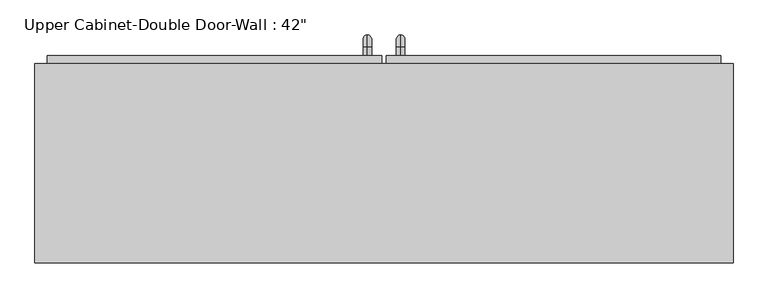
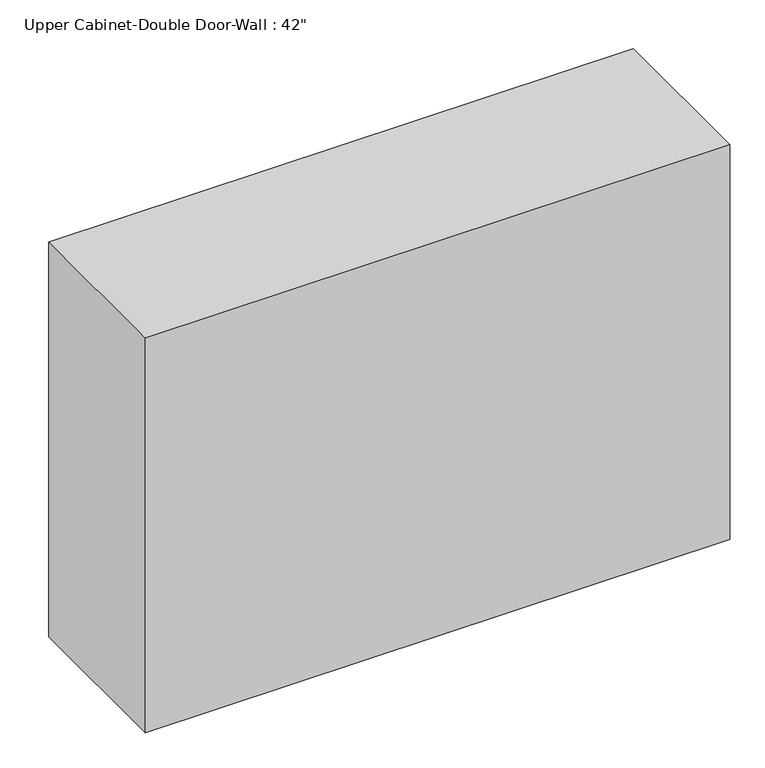
"""IFC4 building model written with IfcOpenShell, lengths in millimetres: furniture geometry."""

from ifc_helpers import new_model, si_unit, point, frame, origin, place, context, project, spatial, polyline, circle_curve, ellipse_curve, trimmed, outline, extrude, faceted_brep, source, transform, mapped, element, save
from ifc_brep_helpers import plane_surface, cylinder_surface, revolved_surface, advanced_brep


def furniture_7e2871f8(model_context):
    return source(origin(), model_context, "Body", "SolidModel", [
        faceted_brep([(-503.6288372, 101.6, 2133.6), (-503.6288372, 101.6, 1371.6), (563.1711628, 101.6, 1371.6), (563.1711628, 101.6, 2133.6), (-503.6288372, 406.4, 2133.6), (563.1711628, 406.4, 2133.6), (563.1711628, 406.4, 1371.6), (-503.6288372, 406.4, 1371.6), (-484.5788372, 406.4, 2114.55), (-484.5788372, 406.4, 1390.65), (544.1211628, 406.4, 1390.65), (544.1211628, 406.4, 2114.55), (544.1211628, 120.65, 2114.55), (-484.5788372, 120.65, 2114.55), (544.1211628, 120.65, 1390.65), (-484.5788372, 120.65, 1390.65)], [[[0, 1, 2, 3]], [[4, 5, 6, 7], [8, 9, 10, 11]], [[1, 0, 4, 7]], [[2, 1, 7, 6]], [[3, 2, 6, 5]], [[0, 3, 5, 4]], [[8, 11, 12, 13]], [[11, 10, 14, 12]], [[10, 9, 15, 14]], [[9, 8, 13, 15]], [[13, 12, 14, 15]]]),
        advanced_brep(
        [(55.1711628, 419.1, 1517.65), (55.1711628, 419.1, 1530.35), (55.1711628, 431.8, 1517.65), (55.1711628, 431.8, 1530.35), (55.1711628, 450.85, 1511.3), (55.1711628, 438.15, 1511.3), (55.1711628, 438.15, 1435.1), (55.1711628, 450.85, 1435.1), (55.1711628, 431.8, 1416.05), (55.1711628, 431.8, 1428.75), (55.1711628, 419.1, 1428.75), (55.1711628, 419.1, 1416.05)],
        [
            (0, 1, circle_curve(frame((55.1711628, 419.1, 1524.0), z_axis=(0.0, -1.0, 0.0), x_axis=(0.0, 0.0, -1.0)), 6.35)),
            (1, 0, circle_curve(frame((55.1711628, 419.1, 1524.0), z_axis=(0.0, -1.0, 0.0), x_axis=(0.0, 0.0, -1.0)), 6.35)),
            (0, 2),
            (2, 3, circle_curve(frame((55.1711628, 431.8, 1524.0), z_axis=(0.0, -1.0, 0.0), x_axis=(0.0, 0.0, -1.0)), 6.35)),
            (3, 1),
            (3, 2, circle_curve(frame((55.1711628, 431.8, 1524.0), z_axis=(0.0, -1.0, 0.0), x_axis=(0.0, 0.0, -1.0)), 6.35)),
            (4, 3, circle_curve(frame((55.1711628, 431.8, 1511.3), z_axis=(1.0, 0.0, 0.0), x_axis=(0.0, 0.0, 1.0)), 19.05)),
            (2, 5, circle_curve(frame((55.1711628, 431.8, 1511.3), z_axis=(-1.0, 0.0, 0.0), x_axis=(0.0, 0.0, 1.0)), 6.35)),
            (5, 4, circle_curve(frame((55.1711628, 444.5, 1511.3), z_axis=(0.0, 0.0, 1.0), x_axis=(0.0, -1.0, 0.0)), 6.35)),
            (4, 5, circle_curve(frame((55.1711628, 444.5, 1511.3), z_axis=(0.0, 0.0, 1.0), x_axis=(0.0, -1.0, 0.0)), 6.35)),
            (5, 6),
            (6, 7, circle_curve(frame((55.1711628, 444.5, 1435.1), z_axis=(0.0, 0.0, 1.0), x_axis=(0.0, -1.0, 0.0)), 6.35)),
            (7, 4),
            (7, 6, circle_curve(frame((55.1711628, 444.5, 1435.1), z_axis=(0.0, 0.0, 1.0), x_axis=(0.0, -1.0, 0.0)), 6.35)),
            (8, 7, circle_curve(frame((55.1711628, 431.8, 1435.1), z_axis=(1.0, 0.0, 0.0), x_axis=(0.0, 1.0, 0.0)), 19.05)),
            (6, 9, circle_curve(frame((55.1711628, 431.8, 1435.1), z_axis=(-1.0, 0.0, 0.0), x_axis=(0.0, 1.0, 0.0)), 6.35)),
            (9, 8, circle_curve(frame((55.1711628, 431.8, 1422.4), z_axis=(0.0, 1.0, 0.0), x_axis=(0.0, 0.0, 1.0)), 6.35)),
            (8, 9, circle_curve(frame((55.1711628, 431.8, 1422.4), z_axis=(0.0, 1.0, 0.0), x_axis=(0.0, 0.0, 1.0)), 6.35)),
            (10, 11, circle_curve(frame((55.1711628, 419.1, 1422.4), z_axis=(0.0, -1.0, 0.0), x_axis=(0.0, 0.0, 1.0)), 6.35)),
            (11, 10, circle_curve(frame((55.1711628, 419.1, 1422.4), z_axis=(0.0, -1.0, 0.0), x_axis=(0.0, 0.0, 1.0)), 6.35)),
            (9, 10),
            (11, 8),
        ],
        [
            plane_surface(frame((48.8211628, 419.1, 1524.0), z_axis=(0.0, -1.0, 0.0), x_axis=(0.0, 0.0, 1.0))),
            cylinder_surface(frame((55.1711628, 419.1, 1524.0), z_axis=(0.0, -1.0, 0.0), x_axis=(0.0, 0.0, -1.0)), 6.35),
            revolved_surface(trimmed(ellipse_curve(frame((55.1711628, 431.8, 1524.0), z_axis=(0.0, -1.0, 0.0), x_axis=(0.0, 0.0, -1.0)), 6.35, 6.35), [point((55.1711628, 431.8, 1517.65))], [point((55.1711628, 431.8, 1530.35))], True, "CARTESIAN"), (55.1711628, 431.8, 1511.3), (-1.0, 0.0, 0.0)),
            revolved_surface(trimmed(ellipse_curve(frame((55.1711628, 431.8, 1524.0), z_axis=(0.0, -1.0, 0.0), x_axis=(0.0, 0.0, -1.0)), 6.35, 6.35), [point((55.1711628, 431.8, 1530.35))], [point((55.1711628, 431.8, 1517.65))], True, "CARTESIAN"), (55.1711628, 431.8, 1511.3), (-1.0, 0.0, 0.0)),
            cylinder_surface(frame((55.1711628, 444.5, 1511.3), z_axis=(0.0, 0.0, 1.0), x_axis=(0.0, -1.0, 0.0)), 6.35),
            revolved_surface(trimmed(ellipse_curve(frame((55.1711628, 444.5, 1435.1), z_axis=(0.0, 0.0, 1.0), x_axis=(0.0, -1.0, 0.0)), 6.35, 6.35), [point((55.1711628, 438.15, 1435.1))], [point((55.1711628, 450.85, 1435.1))], True, "CARTESIAN"), (55.1711628, 431.8, 1435.1), (-1.0, 0.0, 0.0)),
            revolved_surface(trimmed(ellipse_curve(frame((55.1711628, 444.5, 1435.1), z_axis=(0.0, 0.0, 1.0), x_axis=(0.0, -1.0, 0.0)), 6.35, 6.35), [point((55.1711628, 450.85, 1435.1))], [point((55.1711628, 438.15, 1435.1))], True, "CARTESIAN"), (55.1711628, 431.8, 1435.1), (-1.0, 0.0, 0.0)),
            plane_surface(frame((48.8211628, 419.1, 1422.4), z_axis=(0.0, -1.0, 0.0), x_axis=(0.0, 0.0, -1.0))),
            cylinder_surface(frame((55.1711628, 431.8, 1422.4), z_axis=(0.0, 1.0, 0.0), x_axis=(0.0, 0.0, 1.0)), 6.35),
        ],
        [
            (0, [[1, 2]]),
            (1, [[-1, 3, 4, 5]]),
            (1, [[-2, -5, 6, -3]]),
            (2, [[7, -4, 8, 9]]),
            (3, [[-8, -6, -7, 10]]),
            (4, [[-9, 11, 12, 13]]),
            (4, [[-10, -13, 14, -11]]),
            (5, [[15, -12, 16, 17]]),
            (6, [[-16, -14, -15, 18]]),
            (7, [[19, 20]]),
            (8, [[-17, 21, -20, 22]]),
            (8, [[-18, -22, -19, -21]]),
        ],
    ),
        advanced_brep(
        [(4.3711628, 419.1, 1517.65), (4.3711628, 419.1, 1530.35), (4.3711628, 431.8, 1517.65), (4.3711628, 431.8, 1530.35), (4.3711628, 450.85, 1511.3), (4.3711628, 438.15, 1511.3), (4.3711628, 438.15, 1435.1), (4.3711628, 450.85, 1435.1), (4.3711628, 431.8, 1416.05), (4.3711628, 431.8, 1428.75), (4.3711628, 419.1, 1428.75), (4.3711628, 419.1, 1416.05)],
        [
            (0, 1, circle_curve(frame((4.3711628, 419.1, 1524.0), z_axis=(0.0, -1.0, 0.0), x_axis=(0.0, 0.0, 1.0)), 6.35)),
            (1, 0, circle_curve(frame((4.3711628, 419.1, 1524.0), z_axis=(0.0, -1.0, 0.0), x_axis=(0.0, 0.0, 1.0)), 6.35)),
            (0, 2),
            (2, 3, circle_curve(frame((4.3711628, 431.8, 1524.0), z_axis=(0.0, -1.0, 0.0), x_axis=(0.0, 0.0, 1.0)), 6.35)),
            (3, 1),
            (3, 2, circle_curve(frame((4.3711628, 431.8, 1524.0), z_axis=(0.0, -1.0, 0.0), x_axis=(0.0, 0.0, 1.0)), 6.35)),
            (4, 3, circle_curve(frame((4.3711628, 431.8, 1511.3), z_axis=(1.0, 0.0, 0.0), x_axis=(0.0, 0.0, 1.0)), 19.05)),
            (2, 5, circle_curve(frame((4.3711628, 431.8, 1511.3), z_axis=(-1.0, 0.0, 0.0), x_axis=(0.0, 0.0, 1.0)), 6.35)),
            (5, 4, circle_curve(frame((4.3711628, 444.5, 1511.3), z_axis=(0.0, 0.0, 1.0), x_axis=(0.0, 1.0, 0.0)), 6.35)),
            (4, 5, circle_curve(frame((4.3711628, 444.5, 1511.3), z_axis=(0.0, 0.0, 1.0), x_axis=(0.0, 1.0, 0.0)), 6.35)),
            (5, 6),
            (6, 7, circle_curve(frame((4.3711628, 444.5, 1435.1), z_axis=(0.0, 0.0, 1.0), x_axis=(0.0, 1.0, 0.0)), 6.35)),
            (7, 4),
            (7, 6, circle_curve(frame((4.3711628, 444.5, 1435.1), z_axis=(0.0, 0.0, 1.0), x_axis=(0.0, 1.0, 0.0)), 6.35)),
            (8, 7, circle_curve(frame((4.3711628, 431.8, 1435.1), z_axis=(1.0, 0.0, 0.0), x_axis=(0.0, 1.0, 0.0)), 19.05)),
            (6, 9, circle_curve(frame((4.3711628, 431.8, 1435.1), z_axis=(-1.0, 0.0, 0.0), x_axis=(0.0, 1.0, 0.0)), 6.35)),
            (9, 8, circle_curve(frame((4.3711628, 431.8, 1422.4), z_axis=(0.0, 1.0, 0.0), x_axis=(0.0, 0.0, -1.0)), 6.35)),
            (8, 9, circle_curve(frame((4.3711628, 431.8, 1422.4), z_axis=(0.0, 1.0, 0.0), x_axis=(0.0, 0.0, -1.0)), 6.35)),
            (10, 11, circle_curve(frame((4.3711628, 419.1, 1422.4), z_axis=(0.0, -1.0, 0.0), x_axis=(0.0, 0.0, -1.0)), 6.35)),
            (11, 10, circle_curve(frame((4.3711628, 419.1, 1422.4), z_axis=(0.0, -1.0, 0.0), x_axis=(0.0, 0.0, -1.0)), 6.35)),
            (9, 10),
            (11, 8),
        ],
        [
            plane_surface(frame((-1.9788372, 419.1, 1524.0), z_axis=(0.0, -1.0, 0.0), x_axis=(0.0, 0.0, 1.0))),
            cylinder_surface(frame((4.3711628, 419.1, 1524.0), z_axis=(0.0, -1.0, 0.0), x_axis=(0.0, 0.0, 1.0)), 6.35),
            revolved_surface(trimmed(ellipse_curve(frame((4.3711628, 431.8, 1524.0), z_axis=(0.0, -1.0, 0.0), x_axis=(0.0, 0.0, 1.0)), 6.35, 6.35), [point((4.3711628, 431.8, 1517.65))], [point((4.3711628, 431.8, 1530.35))], True, "CARTESIAN"), (4.3711628, 431.8, 1511.3), (-1.0, 0.0, 0.0)),
            revolved_surface(trimmed(ellipse_curve(frame((4.3711628, 431.8, 1524.0), z_axis=(0.0, -1.0, 0.0), x_axis=(0.0, 0.0, 1.0)), 6.35, 6.35), [point((4.3711628, 431.8, 1530.35))], [point((4.3711628, 431.8, 1517.65))], True, "CARTESIAN"), (4.3711628, 431.8, 1511.3), (-1.0, 0.0, 0.0)),
            cylinder_surface(frame((4.3711628, 444.5, 1511.3), z_axis=(0.0, 0.0, 1.0), x_axis=(0.0, 1.0, 0.0)), 6.35),
            revolved_surface(trimmed(ellipse_curve(frame((4.3711628, 444.5, 1435.1), z_axis=(0.0, 0.0, 1.0), x_axis=(0.0, 1.0, 0.0)), 6.35, 6.35), [point((4.3711628, 438.15, 1435.1))], [point((4.3711628, 450.85, 1435.1))], True, "CARTESIAN"), (4.3711628, 431.8, 1435.1), (-1.0, 0.0, 0.0)),
            revolved_surface(trimmed(ellipse_curve(frame((4.3711628, 444.5, 1435.1), z_axis=(0.0, 0.0, 1.0), x_axis=(0.0, 1.0, 0.0)), 6.35, 6.35), [point((4.3711628, 450.85, 1435.1))], [point((4.3711628, 438.15, 1435.1))], True, "CARTESIAN"), (4.3711628, 431.8, 1435.1), (-1.0, 0.0, 0.0)),
            plane_surface(frame((-1.9788372, 419.1, 1422.4), z_axis=(0.0, -1.0, 0.0), x_axis=(0.0, 0.0, -1.0))),
            cylinder_surface(frame((4.3711628, 431.8, 1422.4), z_axis=(0.0, 1.0, 0.0), x_axis=(0.0, 0.0, -1.0)), 6.35),
        ],
        [
            (0, [[1, 2]]),
            (1, [[-1, 3, 4, 5]]),
            (1, [[-2, -5, 6, -3]]),
            (2, [[7, -4, 8, 9]]),
            (3, [[-8, -6, -7, 10]]),
            (4, [[-9, 11, 12, 13]]),
            (4, [[-10, -13, 14, -11]]),
            (5, [[15, -12, 16, 17]]),
            (6, [[-16, -14, -15, 18]]),
            (7, [[19, 20]]),
            (8, [[-17, 21, -20, 22]]),
            (8, [[-18, -22, -19, -21]]),
        ],
    ),
        extrude(outline(polyline([(32.9461628, 419.1), (544.1211628, 419.1), (544.1211628, 387.35), (32.9461628, 387.35), (32.9461628, 419.1)])), frame((0.0, 0.0, 1390.65), z_axis=(0.0, 0.0, 1.0), x_axis=(1.0, 0.0, 0.0)), (0.0, 0.0, 1.0), 723.9),
        extrude(outline(polyline([(-484.5788372, 419.1), (26.5961628, 419.1), (26.5961628, 387.35), (-484.5788372, 387.35), (-484.5788372, 419.1)])), frame((0.0, 0.0, 1390.65), z_axis=(0.0, 0.0, 1.0), x_axis=(1.0, 0.0, 0.0)), (0.0, 0.0, 1.0), 723.9),
    ])


if __name__ == "__main__":
    model = new_model("IFC4")
    model_context = context("Model", 3, world=origin())
    ifc_project = project(units=[si_unit("LENGTHUNIT", "METRE", prefix="MILLI")], contexts=[model_context])
    site = spatial("IfcSite", under=ifc_project)
    building = spatial("IfcBuilding", under=site)
    placement = place(None, origin())
    furniture_shape = furniture_7e2871f8(model_context)
    element("IfcFurniture", 1, ObjectType="Upper Cabinet-Double Door-Wall : 42\"", at=placement, inside=building, context=model_context, shape_type="MappedRepresentation", body=[
        mapped(furniture_shape, transform((0.0, 0.0, 0.0), x_axis=(1.0, 0.0, 0.0), y_axis=(0.0, 1.0, 0.0), z_axis=(0.0, 0.0, 1.0))),
    ])
    save(model, "model.ifc")

# Revit data of these elements
# Type "Upper Cabinet-Double Door-Wall : 42\""
#   Assembly Code = "C1030410"
#   Depth = 1' - 0"
#   Height = 2' - 6"
#   Top Of Cabinet = 7' - 0"
#   Width = 3' - 6"
#   Cabinet Material = none
#   Door/Drawer Material = none
#   Handle Material = Cabinets - Handles
#   Default Elevation = 0
# Element 1 (IfcFurniture, "Upper Cabinet-Double Door-Wall : 42\"")
#   Materials on its faces: "Cabinets - Handles", "Cabinets"
# Materials
#   "Cabinets - Handles": class "Metal", colour RGB 57 57 57, transparency 0
#   "Cabinets": colour RGB 249 249 249, transparency 0
